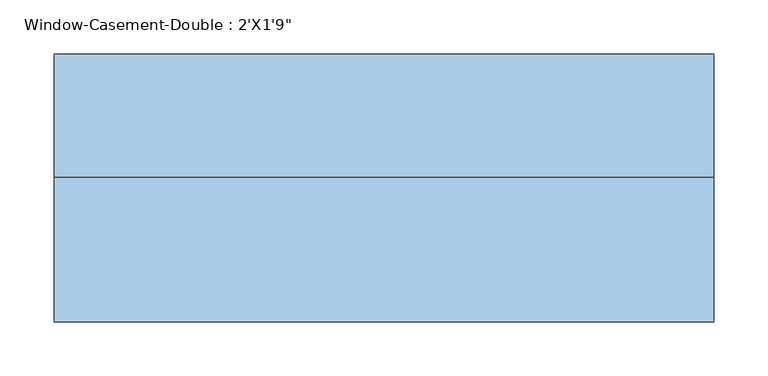
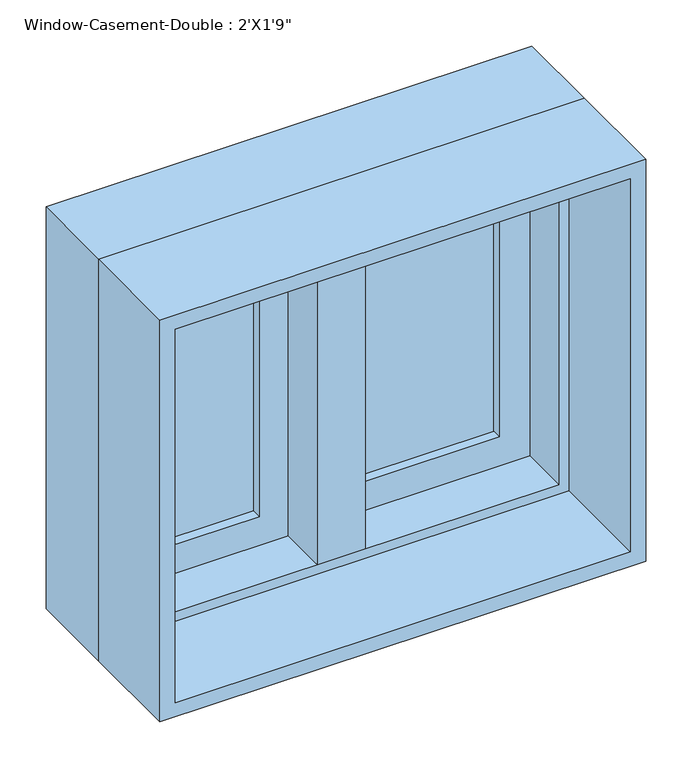
"""IFC4 building model written with IfcOpenShell, lengths in millimetres: window geometry."""

from ifc_helpers import new_model, si_unit, frame, origin, place, context, project, spatial, polyline, outline, extrude, faceted_brep, source, transform, mapped, element, save


def window_79894727(model_context):
    return source(origin(), model_context, "Body", "SolidModel", [
        faceted_brep([(9.525, 133.35, 2654.3), (-9.525, 133.35, 2654.3), (-9.525, 82.55, 2654.3), (9.525, 82.55, 2654.3), (9.525, 133.35, 2146.3), (9.525, 82.55, 2146.3), (-9.525, 82.55, 2146.3), (-9.525, 133.35, 2146.3), (-9.525, 82.55, 2165.35), (-9.525, 82.55, 2635.25), (-30.1625, 82.55, 2165.35), (-30.1625, 82.55, 2635.25), (-30.1625, 19.05, 2165.35), (-30.1625, 19.05, 2635.25), (30.1625, 19.05, 2165.35), (30.1625, 19.05, 2635.25), (30.1625, 82.55, 2165.35), (30.1625, 82.55, 2635.25), (9.525, 82.55, 2165.35), (9.525, 82.55, 2635.25)], [[[0, 1, 2, 3]], [[4, 5, 6, 7]], [[1, 0, 4, 7]], [[2, 1, 7, 6, 8, 9]], [[9, 8, 10, 11]], [[11, 10, 12, 13]], [[13, 12, 14, 15]], [[15, 14, 16, 17]], [[17, 16, 18, 19]], [[0, 3, 19, 18, 5, 4]], [[18, 8, 6, 5]], [[9, 19, 3, 2]], [[8, 18, 16, 14, 12, 10]], [[19, 9, 11, 13, 15, 17]]]),
        extrude(outline(polyline([(-66.675, 114.3), (-66.675, 107.95), (-234.95, 107.95), (-234.95, 114.3), (-66.675, 114.3)])), frame((0.0, 0.0, 2203.45), z_axis=(0.0, 0.0, 1.0), x_axis=(1.0, 0.0, 0.0)), (0.0, 0.0, 1.0), 393.7),
        extrude(outline(polyline([(-234.95, 95.25), (-234.95, 101.6), (-66.675, 101.6), (-66.675, 95.25), (-234.95, 95.25)])), frame((0.0, 0.0, 2203.45), z_axis=(0.0, 0.0, 1.0), x_axis=(1.0, 0.0, 0.0)), (0.0, 0.0, 1.0), 393.7),
        extrude(outline(polyline([(234.95, 114.3), (234.95, 107.95), (66.675, 107.95), (66.675, 114.3), (234.95, 114.3)])), frame((0.0, 0.0, 2203.45), z_axis=(0.0, 0.0, 1.0), x_axis=(1.0, 0.0, 0.0)), (0.0, 0.0, 1.0), 393.7),
        extrude(outline(polyline([(66.675, 95.25), (66.675, 101.6), (234.95, 101.6), (234.95, 95.25), (66.675, 95.25)])), frame((0.0, 0.0, 2203.45), z_axis=(0.0, 0.0, 1.0), x_axis=(1.0, 0.0, 0.0)), (0.0, 0.0, 1.0), 393.7),
        extrude(outline(polyline([(2654.3, -292.1), (2146.3, -292.1), (2146.3, -9.525), (2654.3, -9.525), (2654.3, -292.1)]), holes=[polyline([(2597.15, -66.675), (2203.45, -66.675), (2203.45, -234.95), (2597.15, -234.95), (2597.15, -66.675)])]), frame((0.0, 82.55, 0.0), z_axis=(0.0, 1.0, 0.0), x_axis=(0.0, 0.0, 1.0)), (0.0, 0.0, 1.0), 44.45),
        extrude(outline(polyline([(2146.3, 292.1), (2654.3, 292.1), (2654.3, 9.525), (2146.3, 9.525), (2146.3, 292.1)]), holes=[polyline([(2203.45, 66.675), (2597.15, 66.675), (2597.15, 234.95), (2203.45, 234.95), (2203.45, 66.675)])]), frame((0.0, 82.55, 0.0), z_axis=(0.0, 1.0, 0.0), x_axis=(0.0, 0.0, 1.0)), (0.0, 0.0, 1.0), 44.45),
        extrude(outline(polyline([(2667.0, -304.8), (2133.6, -304.8), (2133.6, 304.8), (2667.0, 304.8), (2667.0, -304.8)]), holes=[polyline([(2647.95, 285.75), (2152.65, 285.75), (2152.65, -285.75), (2647.95, -285.75), (2647.95, 285.75)])]), frame((0.0, -114.3, 0.0), z_axis=(0.0, 1.0, 0.0), x_axis=(0.0, 0.0, 1.0)), (0.0, 0.0, 1.0), 133.35),
        faceted_brep([(273.05, 82.55, 2635.25), (273.05, 19.05, 2635.25), (-273.05, 19.05, 2635.25), (-273.05, 82.55, 2635.25), (292.1, 133.35, 2654.3), (292.1, 82.55, 2654.3), (-292.1, 82.55, 2654.3), (-292.1, 133.35, 2654.3), (304.8, 19.05, 2667.0), (304.8, 133.35, 2667.0), (-304.8, 133.35, 2667.0), (-304.8, 19.05, 2667.0), (-273.05, 19.05, 2165.35), (-273.05, 82.55, 2165.35), (-292.1, 82.55, 2146.3), (-292.1, 133.35, 2146.3), (-304.8, 133.35, 2133.6), (-304.8, 19.05, 2133.6), (273.05, 19.05, 2165.35), (273.05, 82.55, 2165.35), (292.1, 82.55, 2146.3), (292.1, 133.35, 2146.3), (304.8, 133.35, 2133.6), (304.8, 19.05, 2133.6)], [[[0, 1, 2, 3]], [[4, 5, 6, 7]], [[8, 9, 10, 11]], [[3, 2, 12, 13]], [[7, 6, 14, 15]], [[11, 10, 16, 17]], [[13, 12, 18, 19]], [[15, 14, 20, 21]], [[17, 16, 22, 23]], [[11, 17, 23, 8], [1, 18, 12, 2]], [[19, 18, 1, 0]], [[5, 20, 14, 6], [3, 13, 19, 0]], [[21, 20, 5, 4]], [[23, 22, 9, 8]], [[9, 22, 16, 10], [7, 15, 21, 4]]]),
    ])


if __name__ == "__main__":
    model = new_model("IFC4")
    model_context = context("Model", 3, world=origin())
    ifc_project = project(units=[si_unit("LENGTHUNIT", "METRE", prefix="MILLI")], contexts=[model_context])
    site = spatial("IfcSite", under=ifc_project)
    building = spatial("IfcBuilding", under=site)
    placement = place(None, origin())
    window_shape = window_79894727(model_context)
    element("IfcWindow", 1, ObjectType="Window-Casement-Double : 2'X1'9\"", at=placement, inside=building, context=model_context, shape_type="MappedRepresentation", body=[
        mapped(window_shape, transform((0.0, 0.0, 0.0), x_axis=(1.0, 0.0, 0.0), y_axis=(0.0, 1.0, 0.0), z_axis=(0.0, 0.0, 1.0))),
    ])
    save(model, "model.ifc")

# Revit data of these elements
# Type "Window-Casement-Double : 2'X1'9\""
#   Type Mark = "20"
#   Fire Rating = "0.5h"
#   Assembly Code = "B2020100"
#   Analytic Construction = "Double glazing - domestic"
#   Frame Extension [instance default] = 0' - 0 1/4"
#   Window Inset [instance default] = 0' - 0"
#   Wall Thickness [instance default] = 0' - 6"
#   Interior Wall Closure [instance default] = 0' - 2 1/4"
#   Half Width = 1' - 0"
#   Visual Light Transmittance = 0.81
#   Thermal Resistance (R) = 1.8146 (h·ft²·°F)/BTU
#   Solar Heat Gain Coefficient = 0.76
#   Rough Width = 2' - 0 1/2"
#   Rough Height = 1' - 9 1/2"
#   Height = 1' - 9"
#   Heat Transfer Coefficient (U) = 0.5511 BTU/(h·ft²·°F)
#   Exterior Wall Closure [instance default] = 0' - 1 1/4"
#   Extension Jamb [instance default] = 0' - 2 1/4"
#   Default Sill Height = 7' - 0"
#   Width = 2' - 0"
#   Muntin Visibility = yes
#   Interior Trim Visibility [instance default] = yes
#   Exterior Trim Visibility [instance default] = yes
#   Extension Jamb Visibility [instance default] = yes
#   Interior Trim Material = Wood - Stained
#   Muntin Pattern = Muntin Pattern_2x2 : Muntin Pattern_2x2
#   Interior Trim = Trim-Window-Interior-Flat : Picture Frame
#   Interior Frame Material = Wood - Stained
#   Glass Panel Material = Glass
#   Exterior Trim Material = Clad - White
#   Exterior Trim = Trim-Window-Exterior-Flat : with Sill
#   Exterior Frame Material = Clad - White
#   Wall Closure = (empty or 0)
# Element 1 (IfcWindow, "Window-Casement-Double : 2'X1'9\"")
#   Wall Thickness = 0' - 9"
#   Extension Jamb = 0' - 5 1/4"
#   Materials on its faces: "Wood - Stained", "Glass", "Clad - White"
# Materials
#   "Wood - Stained": class "Wood", colour RGB 224 178 126, transparency 0, Cost = 0
#   "Glass": class "Glass", colour RGB 0 128 192, transparency 0.75, Description = "Soda Lime Glass", Cost = 0
#   "Clad - White": class "Wood", colour RGB 242 242 238, transparency 0, Cost = 0
